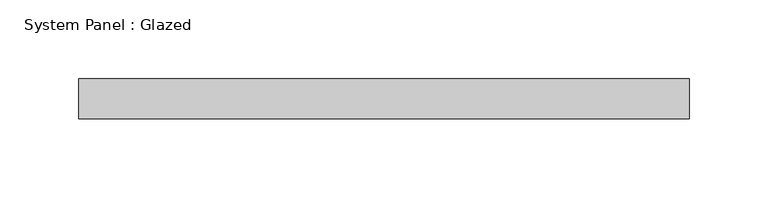
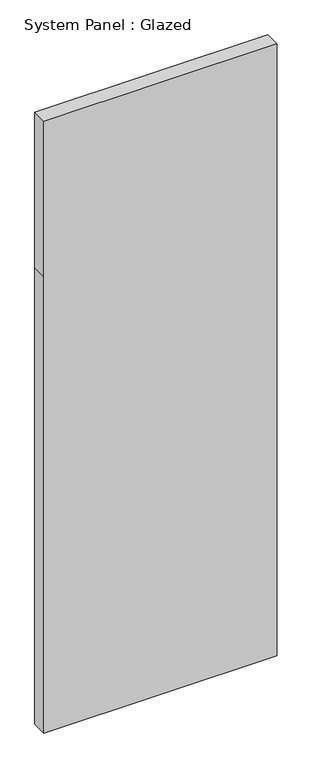
"""IFC4 building model written with IfcOpenShell, lengths in millimetres: plate geometry, System Panel : Glazed."""

from ifc_helpers import new_model, si_unit, frame, origin, place, context, project, spatial, polyline, outline, extrude, source, transform, mapped, element, save


def system_panel_glazed_e6031cb5(model_context):
    return source(origin(), model_context, "Body", "SweptSolid", [
        extrude(outline(polyline([(0.0, -193.675), (0.0, 193.675), (800.1, 193.675), (1073.15, 193.675), (1073.15, -193.675), (800.1, -193.675), (0.0, -193.675)])), frame((0.0, 19.05, 0.0), z_axis=(0.0, 1.0, 0.0), x_axis=(0.0, 0.0, 1.0)), (0.0, 0.0, 1.0), 25.4),
    ])


if __name__ == "__main__":
    model = new_model("IFC4")
    model_context = context("Model", 3, world=origin())
    ifc_project = project(units=[si_unit("LENGTHUNIT", "METRE", prefix="MILLI")], contexts=[model_context])
    site = spatial("IfcSite", under=ifc_project)
    building = spatial("IfcBuilding", under=site)
    placement = place(None, origin())
    system_panel_glazed_shape = system_panel_glazed_e6031cb5(model_context)
    element("IfcPlate", 1, ObjectType="System Panel : Glazed", at=placement, inside=building, context=model_context, shape_type="MappedRepresentation", body=[
        mapped(system_panel_glazed_shape, transform((0.0, 0.0, 0.0), x_axis=(1.0, 0.0, 0.0), y_axis=(0.0, 1.0, 0.0), z_axis=(0.0, 0.0, 1.0))),
    ])
    save(model, "model.ifc")

# Revit data of these elements
# Type "System Panel : Glazed"
#   Construction Type Id = "GSP4R"
#   Analytic Construction = "1/8 in Pilkington single glazing"
#   Visual Light Transmittance = 0.9
#   Solar Heat Gain Coefficient = 0.86
#   Heat Transfer Coefficient (U) = 1.18115 BTU/(h·ft²·°F)
#   Define Thermal Properties by = 1
# Element 1 (IfcPlate, "System Panel : Glazed")
#   Materials on its faces: "Glass"
# Materials
#   "Glass": class "Glass", colour RGB 0 128 192, transparency 0.75, Description = "Soda Lime Glass", Cost = 0
